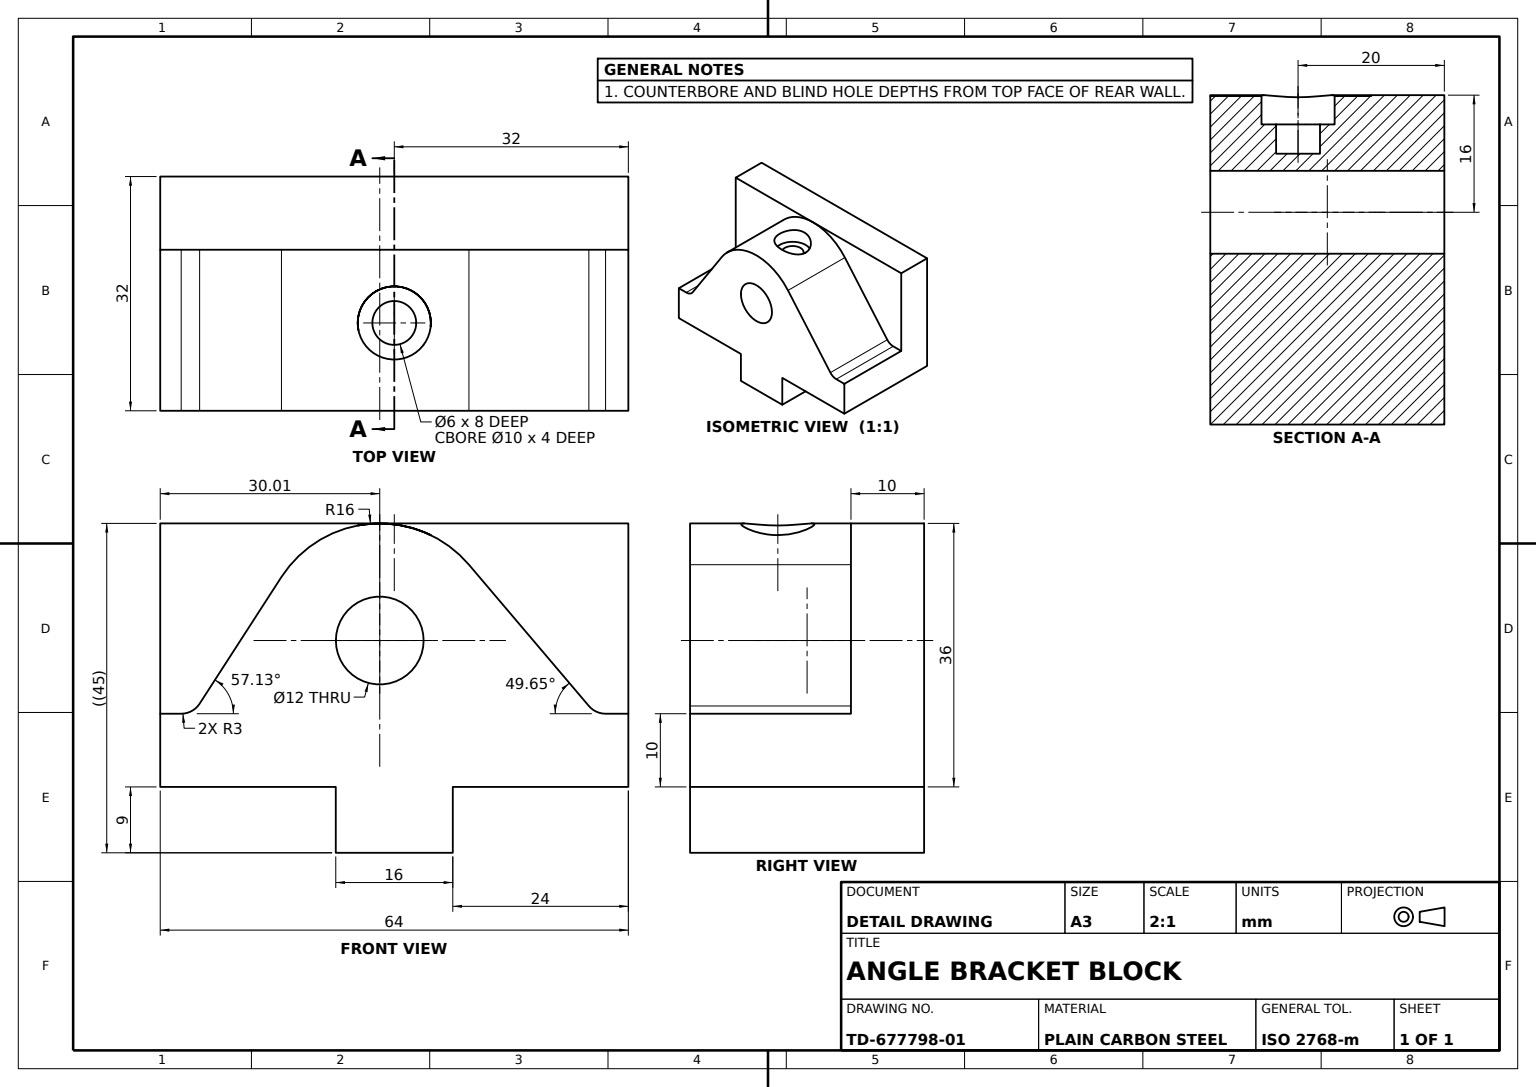
from build123d import *

# Parameters (mm, degrees)
JAW_BODY_DEPTH         = 64
PIVOT_BOSS_DEPTH       = 22
PIVOT_BORE_SKETCH_R    = 6
PIVOT_BORE_12_DEPTH    = 32
GUIDE_KEY_SKETCH_W     = 16
GUIDE_KEY_SKETCH_H     = 9
GUIDE_KEY_DEPTH        = 32
PIVOT_BOSS_FILLET_R3_R = 3
COUNTERBORE_SKETCH_R   = 5
COUNTERBORE_10X4_DEPTH = 4
SCREW_HOLE_SKETCH_R    = 3
SCREW_HOLE_6X4_DEPTH   = 4


with BuildPart() as part:
    # Jaw Body Profile Sketch → Jaw Body (new body)
    with BuildSketch(Plane.XY):
        Polygon((0, 0), (32, 0), (32, 10), (10, 10), (10, 36), (0, 36), align=None)
    extrude(amount=-JAW_BODY_DEPTH)

    # Pivot Boss Sketch → Pivot Boss (add)
    with BuildSketch(Plane(origin=(32, 0, 0), x_dir=(0, 0, -1), z_dir=(1, 0, 0))):
        with BuildLine():
            Line((4.5, 10), (16.574185034, 28.68413566))
            ThreePointArc((16.574185034, 28.68413566), (28.969550727, 35.965977968), (42.206819819, 30.358391585))
            Line((42.206819819, 30.358391585), (59.5, 10))
            Line((59.5, 10), (4.5, 10))
        make_face()
    extrude(amount=-PIVOT_BOSS_DEPTH)

    # Pivot Bore Sketch → Pivot Bore Ø12 (cut)
    with BuildSketch(Plane(origin=(32, 0, 0), x_dir=(0, 0, -1), z_dir=(1, 0, 0))):
        with Locations((30.01240619, 20)):
            Circle(PIVOT_BORE_SKETCH_R)
    extrude(amount=-PIVOT_BORE_12_DEPTH, mode=Mode.SUBTRACT)

    # Guide Key Sketch → Guide Key (add)
    with BuildSketch(Plane(origin=(32, 0, 0), x_dir=(0, 0, -1), z_dir=(1, 0, 0))):
        with Locations((32, -4.5)):
            Rectangle(GUIDE_KEY_SKETCH_W, GUIDE_KEY_SKETCH_H)
    extrude(amount=-GUIDE_KEY_DEPTH)

    # Pivot Boss Fillet R3
    pivot_boss_fillet_r3_edges = [part.edges().sort_by_distance(p)[0] for p in [
        (21, 10, -59.5),
        (21, 10, -4.5),
    ]]
    fillet(pivot_boss_fillet_r3_edges, radius=PIVOT_BOSS_FILLET_R3_R)

    # Counterbore Sketch → Counterbore Ø10x4 (cut)
    with BuildSketch(Plane(origin=(0, 36, 0), x_dir=(1, 0, 0), z_dir=(0, 1, 0))):
        with Locations(Location((20, 32, 0), (0, 0, 270))):
            Circle(COUNTERBORE_SKETCH_R)
    extrude(amount=-COUNTERBORE_10X4_DEPTH, mode=Mode.SUBTRACT)

    # Screw Hole Sketch → Screw Hole Ø6x4 (cut)
    with BuildSketch(Plane(origin=(0, 32, 0), x_dir=(1, 0, 0), z_dir=(0, 1, 0))):
        with Locations(Location((20, 32, 0), (0, 0, 270))):
            Circle(SCREW_HOLE_SKETCH_R)
    extrude(amount=-SCREW_HOLE_6X4_DEPTH, mode=Mode.SUBTRACT)


solid = part.part
